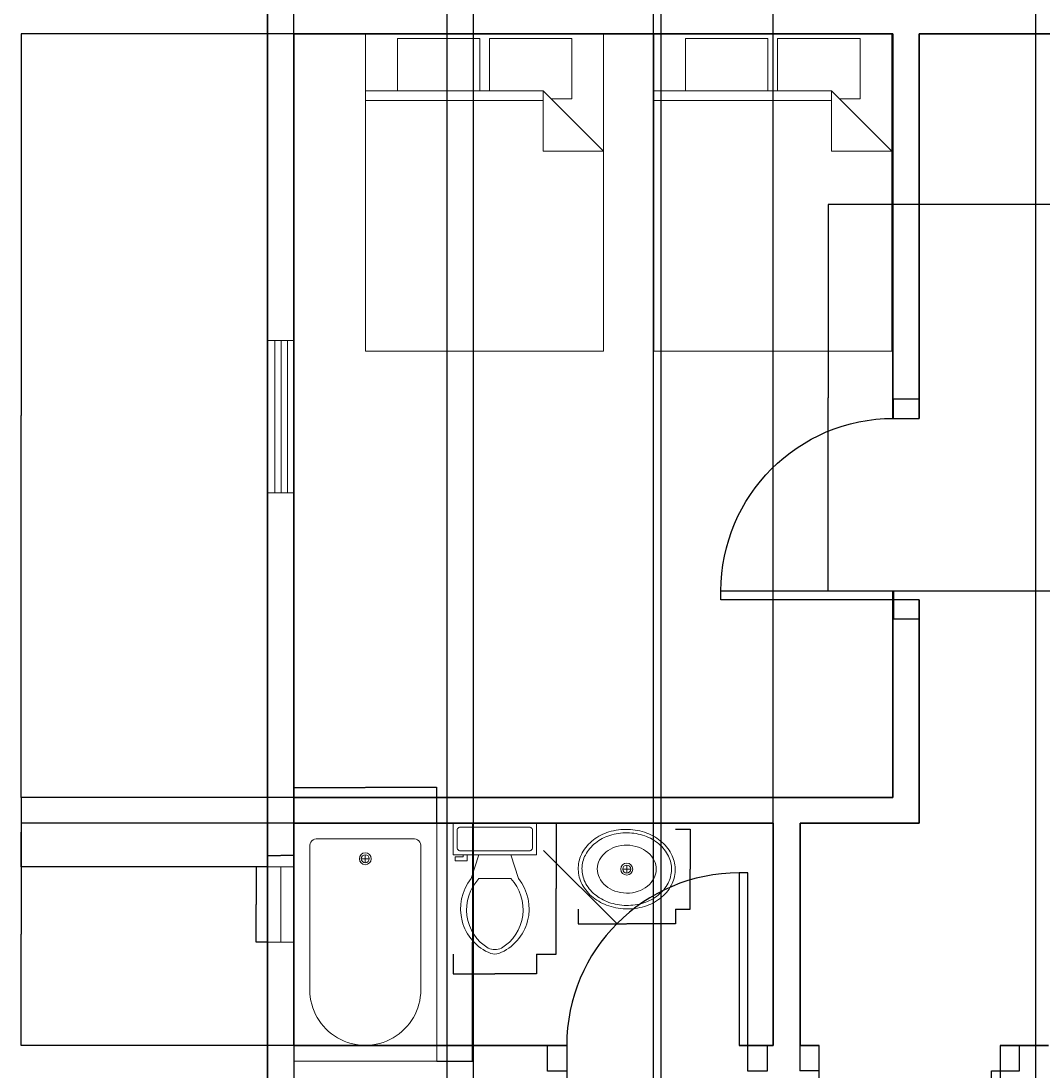
# Model space of a CAD drawing. Units: millimetres. Extents: x 31 to 27050, y -916 to 32407.
# Tile 2 of 7: x 31 to 6569, y 5664 to 12384. Entities that reach past the tile are written whole.
import ezdxf

# ---------------------------------------------------------------- set-up
doc = ezdxf.new("R2010")
doc.units = ezdxf.units.MM
for name, color, linetype, lineweight in [('A-ANNO-DIMS', 2, 'Continuous', 18), ('A-DOOR', 3, 'Continuous', 25), ('A-FLOR-FIXT', 9, 'Continuous', 18), ('A-FURN', 8, 'Continuous', 13), ('A-GLAZ', 4, 'Continuous', 18), ('A-WALL', 7, 'Continuous', 35)]:
    doc.layers.add(name, color=color, linetype=linetype, lineweight=lineweight)
doc.styles.get("Standard").update_dxf_attribs({"font": 'arial.ttf'})
doc.dimstyles.get("Standard").update_dxf_attribs({"dimtxt": 0.18, "dimasz": 0.18, "dimexe": 0.18, "dimexo": 0.0625, "dimgap": 0.09, "dimtad": 0, "dimtih": 1, "dimtoh": 1, "dimdec": 4, "dimzin": 0, "dimdsep": 46, "dimtxsty": 'Standard', "dimcen": 0.09, "dimadec": 0, "dimazin": 0, "dimtfac": 1, "dimtdec": 4, "dimtofl": 0, "dimtmove": 0, "dimatfit": 3, "dimfxl": 1, "dimtolj": 1, "dimtzin": 0, "dimarcsym": 0})

# ---------------------------------------------------------------- blocks, each defined once
blk = doc.blocks.new('Bath Tub - 26 x 60 in.')
for p, q in [((8, -18), (10, -18)), ((9, -17), (9, -19))]:
    blk.add_line(p, q)
blk.add_lwpolyline([(0, -36), (0, 0), (60, 0), (60, -36)], close=True)
for points in [[(6, -4), (42, -4)], [(4, -30), (4, -6)], [(42, -32), (6, -32)]]:
    blk.add_lwpolyline(points)
for radius in [1.5, 1]:
    blk.add_circle((9, -18), radius)
for centre, radius, start, end in [((5.75, -5.75), 1.767766999999999, 81.86989999999999, 188.1301), ((42, -18), 14, 270, 90), ((5.75, -30.25), 1.767766999999999, 171.8699, 278.1301)]:
    blk.add_arc(centre, radius, start, end)
blk = doc.blocks.new('Sink - Oval top')
for p, q in [((-1, 0), (1, 0)), ((0, 1), (0, -1))]:
    blk.add_line(p, q)
for points in [[(-12.23371880354079, 0.3941914712607968, 0.1176342565883263), (-11.46456229543957, -3.361933235489118, 0.104469279667093), (-8.878748691070427, -6.803541973650567, 0.0900157896014849), (-5.082757700676665, -9.072309807490512, 0.0819199491592185), (-0.3227280122732736, -10.01585280257211, 0.0819199491592091), (4.488169920880977, -9.380701564817912, 0.0900157896014801), (8.422342359155778, -7.36101289847943, 0.1044692796670922), (11.22435122606941, -4.093009071543406, 0.1176342565883338), (12.23371880354091, -0.3941914712607968, 0.1176342565883057), (11.46456229543992, 3.361933235488777, 0.1044692796670849), (8.878748691070427, 6.803541973650567, 0.0900157896014884), (5.082757700676324, 9.072309807490681, 0.0819199491592058), (0.3227280122732736, 10.01585280257211, 0.081919949159207), (-4.488169920880864, 9.380701564817969, 0.0900157896014802), (-8.422342359155778, 7.36101289847943, 0.1044692796670951), (-11.22435122606919, 4.093009071543633, 0.1176342565883402)], [(-11.28627986850119, 0.1590597164737346, 0.1186217001864142), (-10.51590095791209, -3.253161772358112, 0.1046781721811095), (-8.071803350560115, -6.358618019863342, 0.0895620664691738), (-4.537699193222351, -8.366971929609804, 0.0811846988912177), (-0.1289739026695997, -9.15150355811437, 0.0811846988912276), (4.300109150126218, -8.491524865184601, 0.0895620664691798), (7.889406708212618, -6.583562428127606, 0.1046781721811044), (10.42004782883111, -3.548216131892445, 0.1186217001864013), (11.28627986850119, -0.1590597164736209, 0.1186217001863945), (10.51590095791221, 3.253161772357998, 0.1046781721811069), (8.071803350560115, 6.358618019863342, 0.0895620664691756), (4.537699193222124, 8.366971929609917, 0.081184698891216), (0.1289739026695997, 9.151503558114428, 0.0811846988912142), (-4.300109150125877, 8.491524865184829, 0.0895620664691747), (-7.889406708212618, 6.583562428127606, 0.1046781721811045), (-10.42004782883111, 3.548216131892445, 0.1186217001863946)], [(-7.420452389032902, 0.0829876781601797, 0.1182825673856775), (-6.907065465214486, -2.1674649380775, 0.1046074595377274), (-5.294791470712084, -4.209988192029413, 0.0897179636260996), (-2.966599981142508, -5.528122152688069, 0.0814360825277113), (-0.0675135187855176, -6.036810076758797, 0.0814360825277218), (2.84222437824053, -5.593085960977873, 0.0897179636261315), (5.199312936802016, -4.327350491993342, 0.1046074595376878), (6.85686365682659, -2.321395784920355, 0.1182825673856714), (7.420452389033016, -0.0829876781601797, 0.1182825673856961), (6.907065465214486, 2.167464938077614, 0.1046074595377135), (5.294791470712084, 4.209988192029413, 0.0897179636261265), (2.966599981142621, 5.528122152687842, 0.0814360825277426), (0.0675135187855176, 6.036810076758797, 0.0814360825277225), (-2.842224378240644, 5.593085960977873, 0.0897179636261212), (-5.199312936802016, 4.327350491993342, 0.1046074595377049), (-6.856863656826476, 2.321395784920355, 0.1182825673856712)]]:
    blk.add_lwpolyline(points, format="xyb", close=True)
for radius in [1.5, 1]:
    blk.add_circle((0, 0), radius)
blk = doc.blocks.new('Toilet - top')
for p, q in [((9.5, -6), (9.5, -2)), ((-10, -8.5), (-8, -8.5)), ((-10, -9.5), (-10, -8.5)), ((-7, -9.5), (-10, -9.5)), ((-8, -8.5), (-8, -8)), ((-7, -8), (-7, -9.5)), ((-4, -8), (-6, -14)), ((4, -8), (6, -14)), ((4, -14), (-4, -14))]:
    blk.add_line(p, q)
blk.add_lwpolyline([(10.5, -8), (10.5, 0), (-10.5, 0), (-10.5, -8)], close=True)
for points in [[(-9.5, -2), (-9.5, -6)], [(8.5, -1), (-8.5, -1)], [(-8.5, -7), (8.5, -7)]]:
    blk.add_lwpolyline(points)
for centre, radius, start, end in [((-8.625, -1.875), 0.8838834999999999, 81.86989999999999, 188.1301), ((8.625, -1.875), 0.8838834999999999, 351.8699, 98.13009999999998), ((-8.625, -6.125), 0.8838834999999999, 171.869898, 278.1301), ((8.625, -6.125), 0.8838834999999999, 261.8699, 8.130099999999993), ((3.519562435188956, -21.58049502388982), 12.16902005083646, 141.4691096810948, 247.9714346835576), ((4.199957580658807, -21.81740929088453), 11.3291791325804, 136.3677254423718, 238.946823937405), ((-3.519499936778316, -21.58047137067522), 12.16903423757823, 292.0284332733152, 38.53070636800453), ((-4.199890672038477, -21.81738596564128), 11.32918622148567, 301.0530065773863, 43.63209216694732), ((2.09660981727e-05, -27.87646475467881), 4, 245.7318247449371, 294.2681740488959), ((2.09415214183e-05, -28.99996806116075), 4, 254.8605283244437, 285.1394707718433)]:
    blk.add_arc(centre, radius, start, end)
blk = doc.blocks.new('Bed - Queen')
for p, q in [((0, -80.00003000000002), (0, 0)), ((0, 0), (59.99998999999999, 0)), ((59.99998999999999, 0), (59.99998999999999, -80.00003000000002)), ((7.99999, -1.200000000000017), (28.79998, -1.200000000000017)), ((7.99999, -14.4), (7.99999, -1.200000000000017)), ((28.79998, -1.200000000000017), (28.79998, -14.4)), ((31.19999, -1.200000000000017), (51.99999000000001, -1.200000000000017)), ((31.19999, -14.4), (31.19999, -1.200000000000017)), ((51.99999000000001, -1.200000000000017), (51.99999000000001, -16.4)), ((0, -14.4), (44.79999999999999, -14.4)), ((59.99998999999999, -29.60000000000001), (44.79999999999999, -14.4)), ((44.79999999999999, -14.4), (44.79999999999999, -29.60000000000001)), ((44.79999999999999, -16.80000000000001), (0, -16.80000000000001)), ((51.99999000000001, -16.4), (46.79936, -16.4)), ((44.79999999999999, -29.60000000000001), (59.99998999999999, -29.60000000000001)), ((59.99998999999999, -80.00003000000002), (0, -80.00003000000002))]:
    blk.add_line(p, q)
blk = doc.blocks.new('Window - Wood Frame 36 in. Wide plan')
for p, q in [((0, 6), (0, 0)), ((36, 6), (36, 0)), ((0, 4.5), (36, 4.5)), ((0, 3), (36, 3)), ((0, 1.5), (36, 1.5))]:
    blk.add_line(p, q)
blk = doc.blocks.new('DOOR-SINGLE-1104')
for p, q in [((56.41678681898429, 1104.337341461596), (-7.18501e-11, 1104.337341461596)), ((-7.18501e-11, 1104.337341461596), (-7.18501e-11, 3.638e-12)), ((56.41678681898429, 7.276e-12), (56.41678681898429, 1104.337341461596)), ((-1226.913698425656, -163.8831223050438), (-1226.913698425656, 3.638e-12)), ((-1104.337341461589, 3.638e-12), (-1226.913698425656, 7.276e-12)), ((-1104.337341461589, 3.638e-12), (-1104.337341461589, -163.8831223050438)), ((-7.18501e-11, 3.638e-12), (56.41678681898429, 7.276e-12)), ((56.41678681898429, -163.8831223050438), (56.41678681898429, 3.638e-12)), ((56.41678681898429, 3.638e-12), (178.9931437830519, 3.638e-12)), ((178.9931437830519, 3.638e-12), (178.9931437830519, -163.8831223050438)), ((-1104.337341461589, -163.8831223050438), (-1226.913698425656, -163.8831223050438)), ((178.9931437830519, -163.8831223050438), (56.41678681898429, -163.8831223050438))]:
    blk.add_line(p, q)
blk.add_arc((0, 3.638e-12), 1104.337341461589, 90, 180)
blk = doc.blocks.new('WIN-BATH-482-FRAMED')
for p, q in [((-2.274e-13, -9.095e-13), (-168.3506507106942, -9.095e-13)), ((-168.3506507106942, -9.095e-13), (-168.3506507106942, -482.3297634273203)), ((-84.17532535534656, -482.3297634273203), (-84.17532535534723, -9.095e-13)), ((-168.3506507106942, -482.3297634273203), (1.1369e-12, -482.3297634273195)), ((1.1369e-12, -482.3297634273195), (-84.17532535534656, -482.3297634273203))]:
    blk.add_line(p, q)
blk = doc.blocks.new('*D22')
at = {"layer": 'A-ANNO-DIMS', "color": 0, "lineweight": -2, "transparency": 16777216}
for p, q in [((2692.835147825165, 7250.543705129638), (2921.552647825165, 7250.543705129638)), ((2921.372647825165, 7250.363705129638), (2921.372647825165, 6488.725608267428)), ((2921.372647825165, 5726.723705129637), (2921.372647825165, 6488.361801991849)), ((2692.835147825164, 5726.543705129636), (2921.552647825165, 5726.543705129636))]:
    blk.add_line(p, q, dxfattribs=at)
at = {"layer": 'A-ANNO-DIMS', "color": 0, "transparency": 16777216}
for points in [[(2921.342647825165, 7250.363705129638), (2921.402647825165, 7250.363705129638), (2921.372647825165, 7250.543705129638)], [(2921.342647825165, 5726.723705129637), (2921.402647825166, 5726.723705129637), (2921.372647825165, 5726.543705129636)]]:
    blk.add_solid(points, dxfattribs=at)
at = {"layer": 'Defpoints', "color": 0, "transparency": 16777216}
for p in [(2692.772647825165, 7250.543705129638), (2692.772647825164, 5726.543705129636), (2921.372647825165, 5726.543705129636)]:
    blk.add_point(p, dxfattribs=at)
at = {"layer": 'A-ANNO-DIMS', "color": 0, "transparency": 16777216, "insert": (2921.372647825167, 6488.543705129636), "char_height": 0.18, "attachment_point": 5}
blk.add_mtext('\\A1;TUB 1524 TYP.', dxfattribs=at)
blk = doc.blocks.new('*D23')
at = {"layer": 'A-ANNO-DIMS', "color": 0, "lineweight": -2, "transparency": 16777216}
for p, q in [((1778.372647825164, 7250.606205129635), (1778.372647825164, 7479.323705129636)), ((1778.552647825164, 7479.143705129636), (2234.974632818343, 7479.143705129636)), ((2692.592647825164, 7479.143705129636), (2236.170662831986, 7479.143705129636)), ((2692.772647825164, 7250.606205129635), (2692.772647825164, 7479.323705129636))]:
    blk.add_line(p, q, dxfattribs=at)
at = {"layer": 'A-ANNO-DIMS', "color": 0, "transparency": 16777216}
for points in [[(1778.552647825164, 7479.173705129635), (1778.552647825164, 7479.113705129636), (1778.372647825164, 7479.143705129636)], [(2692.592647825164, 7479.173705129635), (2692.592647825164, 7479.113705129636), (2692.772647825164, 7479.143705129636)]]:
    blk.add_solid(points, dxfattribs=at)
at = {"layer": 'Defpoints', "color": 0, "transparency": 16777216}
for p in [(2692.772647825164, 7479.143705129636), (1778.372647825164, 7250.543705129635), (2692.772647825164, 7250.543705129635)]:
    blk.add_point(p, dxfattribs=at)
at = {"layer": 'A-ANNO-DIMS', "color": 0, "transparency": 16777216, "insert": (2235.572647825164, 7479.143705129636), "char_height": 0.18, "attachment_point": 5}
blk.add_mtext('\\A1;914 TYP.', dxfattribs=at)
blk = doc.blocks.new('*D24')
at = {"layer": 'A-ANNO-DIMS', "color": 0, "lineweight": -2, "transparency": 16777216}
for p, q in [((3598.273899107064, 6699.857202883667), (3598.273899107064, 6606.20079617063)), ((4221.866610527318, 6699.857202883667), (4221.866610527318, 6606.20079617063)), ((3598.453899107064, 6606.38079617063), (3909.063986058665, 6606.38079617063)), ((4221.686610527318, 6606.38079617063), (3911.076523575718, 6606.38079617063))]:
    blk.add_line(p, q, dxfattribs=at)
at = {"layer": 'A-ANNO-DIMS', "color": 0, "transparency": 16777216}
for points in [[(3598.453899107064, 6606.41079617063), (3598.453899107064, 6606.35079617063), (3598.273899107064, 6606.38079617063)], [(4221.686610527318, 6606.41079617063), (4221.686610527318, 6606.35079617063), (4221.866610527318, 6606.38079617063)]]:
    blk.add_solid(points, dxfattribs=at)
at = {"layer": 'Defpoints', "color": 0, "transparency": 16777216}
for p in [(3598.273899107064, 6699.919702883668), (4221.866610527318, 6699.919702883668), (4221.866610527318, 6606.38079617063)]:
    blk.add_point(p, dxfattribs=at)
at = {"layer": 'A-ANNO-DIMS', "color": 0, "transparency": 16777216, "insert": (3910.070254817191, 6606.38079617063), "char_height": 0.18, "attachment_point": 5}
blk.add_mtext('\\A1;BASIN 624 TYP.', dxfattribs=at)
blk = doc.blocks.new('*D25')
at = {"layer": 'A-ANNO-DIMS', "color": 0, "lineweight": -2, "transparency": 16777216}
for p, q in [((4221.92911052732, 7211.389116326902), (4315.585517240361, 7211.389116326902)), ((4315.40551724036, 7211.209116326902), (4315.40551724036, 6955.836312743077)), ((4315.40551724036, 6700.099702883672), (4315.40551724036, 6955.472506467497)), ((4221.92911052732, 6699.919702883672), (4315.585517240361, 6699.919702883672))]:
    blk.add_line(p, q, dxfattribs=at)
at = {"layer": 'A-ANNO-DIMS', "color": 0, "transparency": 16777216}
for points in [[(4315.375517240361, 7211.209116326902), (4315.43551724036, 7211.209116326902), (4315.40551724036, 7211.389116326902)], [(4315.375517240361, 6700.099702883672), (4315.43551724036, 6700.099702883672), (4315.40551724036, 6699.919702883672)]]:
    blk.add_solid(points, dxfattribs=at)
at = {"layer": 'Defpoints', "color": 0, "transparency": 16777216}
for p in [(4221.86661052732, 7211.389116326902), (4315.40551724036, 7211.389116326902), (4221.86661052732, 6699.919702883672)]:
    blk.add_point(p, dxfattribs=at)
at = {"layer": 'A-ANNO-DIMS', "color": 0, "transparency": 16777216, "insert": (4315.405517240361, 6955.654409605284), "char_height": 0.18, "attachment_point": 5}
blk.add_mtext('\\A1;511 TYP.', dxfattribs=at)
blk = doc.blocks.new('*D26')
at = {"layer": 'A-ANNO-DIMS', "color": 0, "lineweight": -2, "transparency": 16777216}
for p, q in [((3332.083189867999, 7250.543705129638), (3458.106880059174, 7250.543705129638)), ((3457.926880059174, 7250.363705129638), (3457.926880059175, 6831.039535461012)), ((3457.926880059175, 6411.349103855144), (3457.926880059175, 6830.673273523768)), ((3332.083189867999, 6411.169103855144), (3458.106880059175, 6411.169103855144))]:
    blk.add_line(p, q, dxfattribs=at)
at = {"layer": 'A-ANNO-DIMS', "color": 0, "transparency": 16777216}
for points in [[(3457.896880059174, 7250.363705129638), (3457.956880059175, 7250.363705129638), (3457.926880059174, 7250.543705129638)], [(3457.896880059175, 6411.349103855144), (3457.956880059175, 6411.349103855144), (3457.926880059175, 6411.169103855144)]]:
    blk.add_solid(points, dxfattribs=at)
at = {"layer": 'Defpoints', "color": 0, "transparency": 16777216}
for p in [(3332.020689867999, 7250.543705129638), (3457.926880059174, 7250.543705129638), (3332.020689867999, 6411.169103855144)]:
    blk.add_point(p, dxfattribs=at)
at = {"layer": 'A-ANNO-DIMS', "color": 0, "transparency": 16777216, "insert": (3457.926880059176, 6830.856404492388), "char_height": 0.18, "attachment_point": 5}
blk.add_mtext('\\A1;WC 839 TYP.', dxfattribs=at)
blk = doc.blocks.new('*D27')
at = {"layer": 'A-ANNO-DIMS', "color": 0, "lineweight": -2, "transparency": 16777216}
for p, q in [((2798.620689867997, 6411.10660385514), (2798.620689867997, 6285.082913663965)), ((3332.020689867997, 6411.10660385514), (3332.020689867997, 6285.082913663965)), ((2798.800689867997, 6285.262913663966), (3064.722674861176, 6285.262913663966)), ((3331.840689867997, 6285.262913663966), (3065.918704874818, 6285.262913663966))]:
    blk.add_line(p, q, dxfattribs=at)
at = {"layer": 'A-ANNO-DIMS', "color": 0, "transparency": 16777216}
for points in [[(2798.800689867997, 6285.292913663965), (2798.800689867997, 6285.232913663965), (2798.620689867997, 6285.262913663966)], [(3331.840689867997, 6285.292913663965), (3331.840689867997, 6285.232913663965), (3332.020689867997, 6285.262913663966)]]:
    blk.add_solid(points, dxfattribs=at)
at = {"layer": 'Defpoints', "color": 0, "transparency": 16777216}
for p in [(2798.620689867997, 6411.16910385514), (3332.020689867997, 6411.16910385514), (3332.020689867997, 6285.262913663966)]:
    blk.add_point(p, dxfattribs=at)
at = {"layer": 'A-ANNO-DIMS', "color": 0, "transparency": 16777216, "insert": (3065.320689867997, 6285.262913663966), "char_height": 0.18, "attachment_point": 5}
blk.add_mtext('\\A1;533 TYP.', dxfattribs=at)
blk = doc.blocks.new('*D42')
at = {"layer": 'A-ANNO-DIMS', "color": 0, "lineweight": -2, "transparency": 16777216}
for p, q in [((1609.959497114469, 6971.117434470525), (1537.492532600372, 6971.117434470525)), ((1537.672532600373, 6970.937434470525), (1537.672532600373, 6730.135683725489)), ((1537.672532600373, 6488.967671043207), (1537.672532600373, 6729.769421788244)), ((1609.959497114469, 6488.787671043207), (1537.492532600373, 6488.787671043207))]:
    blk.add_line(p, q, dxfattribs=at)
at = {"layer": 'A-ANNO-DIMS', "color": 0, "transparency": 16777216}
for points in [[(1537.642532600373, 6970.937434470525), (1537.702532600373, 6970.937434470525), (1537.672532600373, 6971.117434470525)], [(1537.642532600373, 6488.967671043207), (1537.702532600373, 6488.967671043207), (1537.672532600373, 6488.787671043207)]]:
    blk.add_solid(points, dxfattribs=at)
at = {"layer": 'Defpoints', "color": 0, "transparency": 16777216}
for p in [(1537.672532600373, 6971.117434470525), (1610.021997114469, 6971.117434470525), (1610.021997114469, 6488.787671043207)]:
    blk.add_point(p, dxfattribs=at)
at = {"layer": 'A-ANNO-DIMS', "color": 0, "transparency": 16777216, "insert": (1537.672532600374, 6729.952552756865), "char_height": 0.18, "attachment_point": 5}
blk.add_mtext('\\A1;FRAMED WINDOW 482 TYP.', dxfattribs=at)
blk = doc.blocks.new('*D43')
at = {"layer": 'A-ANNO-DIMS', "color": 0, "lineweight": -2, "transparency": 16777216}
for p, q in [((1610.021997114469, 6971.179934470523), (1610.021997114469, 7043.64689898462)), ((1610.201997114469, 7043.46689898462), (1693.607779495737, 7043.46689898462)), ((1778.192647825164, 7043.46689898462), (1694.786865443895, 7043.46689898462)), ((1778.372647825164, 6971.179934470523), (1778.372647825164, 7043.64689898462))]:
    blk.add_line(p, q, dxfattribs=at)
at = {"layer": 'A-ANNO-DIMS', "color": 0, "transparency": 16777216}
for points in [[(1610.201997114469, 7043.49689898462), (1610.201997114469, 7043.43689898462), (1610.021997114469, 7043.46689898462)], [(1778.192647825164, 7043.49689898462), (1778.192647825164, 7043.43689898462), (1778.372647825164, 7043.46689898462)]]:
    blk.add_solid(points, dxfattribs=at)
at = {"layer": 'Defpoints', "color": 0, "transparency": 16777216}
for p in [(1778.372647825164, 7043.46689898462), (1610.021997114469, 6971.117434470523), (1778.372647825164, 6971.117434470523)]:
    blk.add_point(p, dxfattribs=at)
at = {"layer": 'A-ANNO-DIMS', "color": 0, "transparency": 16777216, "insert": (1694.197322469817, 7043.46689898462), "char_height": 0.18, "attachment_point": 5}
blk.add_mtext('\\A1;168 TYP.', dxfattribs=at)
blk = doc.blocks.new('*D57')
at = {"layer": 'A-ANNO-DIMS', "color": 0, "lineweight": -2, "transparency": 16777216}
for p, q in [((1778.310148000001, 12301.860549), (30.84199699999932, 12301.860549)), ((31.02199699999948, 12301.68054900001), (31.02199700000003, 9858.325591137795)), ((31.02199700000057, 7414.606827000004), (31.02199700000003, 9857.961784862217)), ((1778.310148000001, 7414.426827000004), (30.8419970000004, 7414.426827000004))]:
    blk.add_line(p, q, dxfattribs=at)
at = {"layer": 'A-ANNO-DIMS', "color": 0, "transparency": 16777216}
for points in [[(30.99199699999948, 12301.68054900001), (31.05199699999948, 12301.68054900001), (31.02199699999948, 12301.860549)], [(30.99199700000057, 7414.606827000004), (31.05199700000057, 7414.606827000004), (31.02199700000057, 7414.426827000004)]]:
    blk.add_solid(points, dxfattribs=at)
at = {"layer": 'Defpoints', "color": 0, "transparency": 16777216}
for p in [(31.02199699999948, 12301.860549), (1778.372648000001, 12301.860549), (1778.372648000001, 7414.426827000004)]:
    blk.add_point(p, dxfattribs=at)
at = {"layer": 'A-ANNO-DIMS', "color": 0, "transparency": 16777216, "insert": (31.02199700000281, 9858.143688000006), "char_height": 0.18, "attachment_point": 5}
blk.add_mtext('\\A1;4887', dxfattribs=at)
blk = doc.blocks.new('*D58')
at = {"layer": 'A-ANNO-DIMS', "color": 0, "lineweight": -2, "transparency": 16777216}
for p, q in [((1778.310148000001, 7250.543705000004), (30.84199699999976, 7250.543705000004)), ((31.02199699999987, 7250.363705000004), (31.02199700000003, 6539.219446529336)), ((31.02199700000019, 5827.711259000002), (31.02199700000003, 6538.855517470672)), ((1778.310148000001, 5827.531259000002), (30.84199700000007, 5827.531259000002))]:
    blk.add_line(p, q, dxfattribs=at)
at = {"layer": 'A-ANNO-DIMS', "color": 0, "transparency": 16777216}
for points in [[(30.99199699999987, 7250.363705000004), (31.05199699999988, 7250.363705000004), (31.02199699999987, 7250.543705000004)], [(30.99199700000019, 5827.711259000002), (31.05199700000019, 5827.711259000002), (31.02199700000019, 5827.531259000002)]]:
    blk.add_solid(points, dxfattribs=at)
at = {"layer": 'Defpoints', "color": 0, "transparency": 16777216}
for p in [(31.02199699999987, 7250.543705000004), (1778.372648000001, 7250.543705000004), (1778.372648000001, 5827.531259000002)]:
    blk.add_point(p, dxfattribs=at)
at = {"layer": 'A-ANNO-DIMS', "color": 0, "transparency": 16777216, "insert": (31.02199700000188, 6539.037482000002), "char_height": 0.18, "attachment_point": 5}
blk.add_mtext('\\A1;1423', dxfattribs=at)
blk = doc.blocks.new('*D61')
at = {"layer": 'A-ANNO-DIMS', "color": 0, "lineweight": -2, "transparency": 16777216}
for p, q in [((1778.372648, 7250.606205), (1778.372648000001, 32406.711259)), ((1778.552648000001, 32406.531259), (3312.109331318556, 32406.531259)), ((4846.592413000001, 32406.531259), (3313.035729681448, 32406.531259)), ((4846.772413, 7250.606205), (4846.772413000001, 32406.711259))]:
    blk.add_line(p, q, dxfattribs=at)
at = {"layer": 'A-ANNO-DIMS', "color": 0, "transparency": 16777216}
for points in [[(1778.552648000001, 32406.561259), (1778.552648000001, 32406.501259), (1778.372648000001, 32406.531259)], [(4846.592413000001, 32406.561259), (4846.592413000001, 32406.501259), (4846.772413000001, 32406.531259)]]:
    blk.add_solid(points, dxfattribs=at)
at = {"layer": 'Defpoints', "color": 0, "transparency": 16777216}
for p in [(4846.772413000001, 32406.531259), (1778.372648, 7250.543705), (4846.772413, 7250.543705)]:
    blk.add_point(p, dxfattribs=at)
at = {"layer": 'A-ANNO-DIMS', "color": 0, "transparency": 16777216, "insert": (3312.572530500002, 32406.531259), "char_height": 0.18, "attachment_point": 5}
blk.add_mtext('\\A1;3068.4', dxfattribs=at)
blk = doc.blocks.new('*D64')
at = {"layer": 'A-ANNO-DIMS', "color": 0, "lineweight": -2, "transparency": 16777216}
for p, q in [((6778.040612000004, 11210.336516), (5198.923112000002, 11210.336516)), ((5199.103112000003, 11210.156516), (5199.103112000003, 9972.897271637792)), ((5199.103112000003, 8735.274221000001), (5199.103112000003, 9972.533465362214)), ((6778.040612000004, 8735.094221000001), (5198.923112000003, 8735.094221000001))]:
    blk.add_line(p, q, dxfattribs=at)
at = {"layer": 'A-ANNO-DIMS', "color": 0, "transparency": 16777216}
for points in [[(5199.073112000003, 11210.156516), (5199.133112000002, 11210.156516), (5199.103112000003, 11210.336516)], [(5199.073112000004, 8735.274221000001), (5199.133112000003, 8735.274221000001), (5199.103112000003, 8735.094221000001)]]:
    blk.add_solid(points, dxfattribs=at)
at = {"layer": 'Defpoints', "color": 0, "transparency": 16777216}
for p in [(5199.103112000003, 11210.336516), (6778.103112000003, 11210.336516), (6778.103112000003, 8735.094221000001)]:
    blk.add_point(p, dxfattribs=at)
at = {"layer": 'A-ANNO-DIMS', "color": 0, "transparency": 16777216, "insert": (5199.103112000005, 9972.7153685), "char_height": 0.18, "attachment_point": 5}
blk.add_mtext('\\A1;2475', dxfattribs=at)
blk = doc.blocks.new('*D69')
at = {"layer": 'A-ANNO-DIMS', "color": 0, "lineweight": -2, "transparency": 16777216}
for p, q in [((2757.340836, 14467.362437), (2757.340835999999, -915.5318640000004)), ((4128.594056999999, 14467.362437), (4128.594056999999, -915.5318640000004)), ((2757.520835999999, -915.3518639999999), (3442.512289610504, -915.3518639999999)), ((4128.414056999999, -915.3518639999999), (3443.422603389495, -915.3518639999999))]:
    blk.add_line(p, q, dxfattribs=at)
at = {"layer": 'A-ANNO-DIMS', "color": 0, "transparency": 16777216}
for points in [[(2757.520835999999, -915.321864), (2757.520835999999, -915.381864), (2757.340835999999, -915.3518639999999)], [(4128.414056999999, -915.321864), (4128.414056999999, -915.381864), (4128.594056999999, -915.3518639999999)]]:
    blk.add_solid(points, dxfattribs=at)
at = {"layer": 'Defpoints', "color": 0, "transparency": 16777216}
for p in [(2757.340836, 14467.424937), (4128.594056999999, 14467.424937), (4128.594056999999, -915.3518639999999)]:
    blk.add_point(p, dxfattribs=at)
at = {"layer": 'A-ANNO-DIMS', "color": 0, "transparency": 16777216, "insert": (3442.967446499999, -915.3518639999999), "char_height": 0.18, "attachment_point": 5}
blk.add_mtext('\\A1;1371.3', dxfattribs=at)
blk = doc.blocks.new('*D70')
at = {"layer": 'A-ANNO-DIMS', "color": 0, "lineweight": -2, "transparency": 16777216}
for p, q in [((4128.594056999999, 14467.362437), (4128.594056999999, -915.5318640000004)), ((6528.594057000001, 14467.362437), (6528.594056999999, -915.5318640000004)), ((4128.774057, -915.3518639999999), (5328.234056999999, -915.3518639999999)), ((6528.414056999999, -915.3518639999999), (5328.954056999999, -915.3518639999999))]:
    blk.add_line(p, q, dxfattribs=at)
at = {"layer": 'A-ANNO-DIMS', "color": 0, "transparency": 16777216}
for points in [[(4128.774057, -915.321864), (4128.774057, -915.381864), (4128.594056999999, -915.3518639999999)], [(6528.414056999999, -915.321864), (6528.414056999999, -915.381864), (6528.594056999999, -915.3518639999999)]]:
    blk.add_solid(points, dxfattribs=at)
at = {"layer": 'Defpoints', "color": 0, "transparency": 16777216}
for p in [(4128.594056999999, 14467.424937), (6528.594057000001, 14467.424937), (6528.594056999999, -915.3518639999999)]:
    blk.add_point(p, dxfattribs=at)
at = {"layer": 'A-ANNO-DIMS', "color": 0, "transparency": 16777216, "insert": (5328.594057, -915.3518639999999), "char_height": 0.18, "attachment_point": 5}
blk.add_mtext('\\A1;2400', dxfattribs=at)
blk = doc.blocks.new('*D84')
at = {"layer": 'A-ANNO-DIMS', "color": 0, "lineweight": -2, "transparency": 16777216}
for p, q in [((1778.310148000001, 7414.426827000004), (30.84199699999995, 7414.426827000004)), ((31.02199699999998, 7414.246827000003), (31.02199700000003, 7192.954095029334)), ((31.02199700000008, 6971.297434000004), (31.02199700000003, 7192.590165970671)), ((1609.959497000001, 6971.117434000004), (30.84199700000004, 6971.117434000004))]:
    blk.add_line(p, q, dxfattribs=at)
at = {"layer": 'A-ANNO-DIMS', "color": 0, "transparency": 16777216}
for points in [[(30.99199699999998, 7414.246827000003), (31.05199699999998, 7414.246827000003), (31.02199699999998, 7414.426827000004)], [(30.99199700000008, 6971.297434000004), (31.05199700000008, 6971.297434000004), (31.02199700000008, 6971.117434000004)]]:
    blk.add_solid(points, dxfattribs=at)
at = {"layer": 'Defpoints', "color": 0, "transparency": 16777216}
for p in [(31.02199699999998, 7414.426827000004), (1778.372648000001, 7414.426827000004), (1610.021997000001, 6971.117434000004)]:
    blk.add_point(p, dxfattribs=at)
at = {"layer": 'A-ANNO-DIMS', "color": 0, "transparency": 16777216, "insert": (31.02199700000206, 7192.772130500002), "char_height": 0.18, "attachment_point": 5}
blk.add_mtext('\\A1;443.3', dxfattribs=at)
blk = doc.blocks.new('*D92')
at = {"layer": 'A-ANNO-DIMS', "color": 0, "lineweight": -2, "transparency": 16777216}
for p, q in [((1778.372648, 5827.468759000001), (1778.372647999999, -915.5318640000004)), ((3525.344535, 5827.468759000001), (3525.344535, -915.5318640000004)), ((1778.552647999999, -915.3518639999999), (2651.508291363575, -915.3518639999999)), ((3525.164535, -915.3518639999999), (2652.208891636425, -915.3518639999999))]:
    blk.add_line(p, q, dxfattribs=at)
at = {"layer": 'A-ANNO-DIMS', "color": 0, "transparency": 16777216}
for points in [[(1778.552647999999, -915.321864), (1778.552647999999, -915.381864), (1778.372647999999, -915.3518639999999)], [(3525.164535, -915.321864), (3525.164535, -915.381864), (3525.344535, -915.3518639999999)]]:
    blk.add_solid(points, dxfattribs=at)
at = {"layer": 'Defpoints', "color": 0, "transparency": 16777216}
for p in [(1778.372648, 5827.531259), (3525.344535, 5827.531259), (3525.344535, -915.3518639999999)]:
    blk.add_point(p, dxfattribs=at)
at = {"layer": 'A-ANNO-DIMS', "color": 0, "transparency": 16777216, "insert": (2651.8585915, -915.3518639999999), "char_height": 0.18, "attachment_point": 5}
blk.add_mtext('\\A1;1747', dxfattribs=at)
blk = doc.blocks.new('*D93')
at = {"layer": 'A-ANNO-DIMS', "color": 0, "lineweight": -2, "transparency": 16777216}
for p, q in [((2925.691486, 14303.479314), (2925.691486, -915.5318640000004)), ((4078.94748, 14303.479314), (4078.947479999999, -915.5318640000004)), ((2925.871485999999, -915.3518639999999), (3501.864326110504, -915.3518639999999)), ((4078.767479999998, -915.3518639999999), (3502.774639889495, -915.3518639999999))]:
    blk.add_line(p, q, dxfattribs=at)
at = {"layer": 'A-ANNO-DIMS', "color": 0, "transparency": 16777216}
for points in [[(2925.871485999999, -915.321864), (2925.871485999999, -915.381864), (2925.691486, -915.3518639999999)], [(4078.767479999998, -915.321864), (4078.767479999998, -915.381864), (4078.947479999999, -915.3518639999999)]]:
    blk.add_solid(points, dxfattribs=at)
at = {"layer": 'Defpoints', "color": 0, "transparency": 16777216}
for p in [(2925.691486, 14303.541814), (4078.94748, 14303.541814), (4078.947479999999, -915.3518639999999)]:
    blk.add_point(p, dxfattribs=at)
at = {"layer": 'A-ANNO-DIMS', "color": 0, "transparency": 16777216, "insert": (3502.319482999999, -915.3518639999999), "char_height": 0.18, "attachment_point": 5}
blk.add_mtext('\\A1;1153.3', dxfattribs=at)
blk = doc.blocks.new('*D95')
at = {"layer": 'A-ANNO-DIMS', "color": 0, "lineweight": -2, "transparency": 16777216}
for p, q in [((3377.522847247268, 7074.377110152927), (3377.702847247268, 7074.377110152926)), ((3377.702847247268, 7074.377110152926), (3847.067442586853, 6606.936933490977)), ((4629.591876, 5827.531259000001), (4629.771876, 5827.531259)), ((4629.681876000001, 5827.441259000001), (4629.681875999998, 5827.621259000001))]:
    blk.add_line(p, q, dxfattribs=at)
at = {"layer": 'A-ANNO-DIMS', "color": 0, "transparency": 16777216}
blk.add_solid([(3847.088612168682, 6606.958190226501), (3847.046273005023, 6606.915676755453), (3847.194983000001, 6606.809916)], dxfattribs=at)
at = {"layer": 'Defpoints', "color": 0, "transparency": 16777216}
for p in [(3847.194983000001, 6606.809916), (4629.681876, 5827.531259000001)]:
    blk.add_point(p, dxfattribs=at)
at = {"layer": 'A-ANNO-DIMS', "color": 0, "transparency": 16777216, "insert": (3376.708242881647, 7074.377110152927), "char_height": 0.18, "attachment_point": 5}
blk.add_mtext('\\A1;28X R1104.3', dxfattribs=at)

msp = doc.modelspace()

# ---------------------------------------------------------------- linework, layer by layer
at = {"layer": 'A-DOOR'}
for p, q in [((5617.824553716266, 8556.807120053505), (5781.707676021313, 8556.807120053505)), ((5019.966376369207, 5827.531258671735), (5141.437222462371, 5827.531258671735)), ((6424.767707707011, 5663.648136366686), (6424.767707707011, 5827.531258671734))]:
    msp.add_line(p, q, dxfattribs=at)
at = {"layer": 'A-WALL'}
for p, q in [((1610.021997114469, 744.3803777755929), (1610.021997114469, 12465.74367114627)), ((5613.357025310619, 12301.86054884122), (1778.372647825163, 12301.86054884122)), ((1778.372647825163, 5827.531258671735), (1778.372647825163, 12301.86054884122)), ((5613.357025310619, 12301.86054884122), (5613.357025310619, 9840.128568706263)), ((5781.707676021313, 12301.86054884122), (5781.707676021314, 9840.137605298149)), ((8211.090788713413, 12301.86054884122), (5781.707676021313, 12301.86054884121)), ((5613.357025310619, 8735.80026383663), (5613.357025310619, 7414.426827434685)), ((5781.707676021315, 8679.383477017574), (5781.707676021314, 7331.275946538546)), ((4846.772413104511, 7414.426827434685), (1778.372647825163, 7414.426827434685)), ((4846.772413104511, 7414.426827434685), (4926.421654242644, 7414.426827434687)), ((5613.357025310619, 7414.426827434685), (4926.421654242644, 7414.426827434687)), ((5781.707676021314, 7250.543705129635), (5781.707676021314, 7331.275946538546)), ((4846.772413104511, 7250.543705129635), (1778.372647825163, 7250.543705129636)), ((4846.772413104512, 7250.543705129635), (4846.772413104511, 5827.531258671734)), ((5693.9203608066, 7250.543705129635), (5019.966376369208, 7250.543705129635)), ((5019.966376369208, 7250.543705129635), (5019.966376369208, 5827.531258671735)), ((5693.9203608066, 7250.543705129635), (5781.707676021314, 7250.543705129635)), ((1778.372647825163, 5827.531258671735), (3525.344534980938, 5827.531258671734)), ((4629.681876442453, 5827.531258671734), (4846.772413104512, 5827.531258671734)), ((6302.191350742941, 5827.531258671733), (6610.021997114469, 5827.531258671733))]:
    msp.add_line(p, q, dxfattribs=at)

# ---------------------------------------------------------------- block references
at = {"layer": 'A-DOOR', "extrusion": (0, 0, -1), "zscale": -1}
for p, rotation in [((-5617.82455371628, 8735.800263836558), 270.0000000000002), ((-6245.774563923957, 5663.648136366701), 180)]:
    msp.add_blockref('DOOR-SINGLE-1104', p, dxfattribs=dict(at, rotation=rotation))
at = {"layer": 'A-DOOR'}
msp.add_blockref('DOOR-SINGLE-1104', (4629.681876442521, 5827.531258671719), dxfattribs=at)
at = {"layer": 'A-FLOR-FIXT', "xscale": 25.4, "yscale": 25.4, "zscale": 25.4, "rotation": 270}
msp.add_blockref('Bath Tub - 26 x 60 in.', (2692.772647825164, 7250.543705129635), dxfattribs=at)
at = {"layer": 'A-FLOR-FIXT', "xscale": 25.4, "yscale": 25.4, "zscale": 25.4}
for name, p in [('Toilet - top', (3065.320689867997, 7250.543705129635)), ('Sink - Oval top', (3910.07025481719, 6955.654409605282))]:
    msp.add_blockref(name, p, dxfattribs=at)
at = {"layer": 'A-FURN', "xscale": 25.4, "yscale": 25.4, "zscale": 25.4}
for p in [(2237.698750248645, 12301.86054884122), (4082.975090126507, 12301.86054884122)]:
    msp.add_blockref('Bed - Queen', p, dxfattribs=at)
at = {"layer": 'A-GLAZ', "xscale": 27.11229900122799, "yscale": 27.11229900122799, "zscale": 27.11229900122799, "rotation": 90}
msp.add_blockref('Window - Wood Frame 36 in. Wide plan', (1778.372647825162, 9363.310953655888), dxfattribs=at)
at = {"layer": 'A-GLAZ'}
msp.add_blockref('WIN-BATH-482-FRAMED', (1778.372647825163, 6971.117434470523), dxfattribs=at)

# ---------------------------------------------------------------- dimensions: what is measured, and where the dimension line sits
at = {"layer": 'A-ANNO-DIMS'}
for base, p1, p2, override, picture, middle in [((4846.772413000001, 32406.531259), (1778.372648, 7250.543705), (4846.772413, 7250.543705), {"dimdec": 1, "dimlfac": 1, "dimrnd": 0, "dimzin": 0, "dimdsep": 46, "dimlunit": 2}, '*D61', (3312.572530500002, 32406.531259)), ((4128.594056999999, -915.3518639999999), (2757.340836, 14467.424937), (4128.594056999999, 14467.424937), {"dimdec": 1, "dimlfac": 1, "dimrnd": 0, "dimzin": 0, "dimdsep": 46, "dimlunit": 2}, '*D69', (3442.967446499999, -915.3518639999999)), ((6528.594056999999, -915.3518639999999), (4128.594056999999, 14467.424937), (6528.594057000001, 14467.424937), {"dimdec": 0, "dimlfac": 1, "dimrnd": 0, "dimzin": 0, "dimdsep": 46, "dimlunit": 2}, '*D70', (5328.594057, -915.3518639999999)), ((4078.947479999999, -915.3518639999999), (2925.691486, 14303.541814), (4078.94748, 14303.541814), {"dimdec": 1, "dimlfac": 1, "dimrnd": 0, "dimzin": 0, "dimdsep": 46, "dimlunit": 2}, '*D93', (3502.319482999999, -915.3518639999999)), ((3525.344535, -915.3518639999999), (1778.372648, 5827.531259), (3525.344535, 5827.531259), {"dimdec": 0, "dimlfac": 1, "dimrnd": 0, "dimzin": 0, "dimdsep": 46, "dimlunit": 2}, '*D92', (2651.8585915, -915.3518639999999))]:
    dim = msp.add_linear_dim(base=base, p1=p1, p2=p2, dimstyle='Standard', override=override, dxfattribs=at)
    dim.commit()
    dim.dimension.update_dxf_attribs({"geometry": picture, "text_midpoint": middle})
for base, p1, p2, angle, override, picture, middle in [((31.02199699999948, 12301.860549), (1778.372648, 7414.426826999999), (1778.372648, 12301.860549), 90, {"dimdec": 0, "dimlfac": 1, "dimrnd": 0, "dimzin": 0, "dimdsep": 46, "dimlunit": 2}, '*D57', (31.02199700000281, 9858.143688000006)), ((5199.103112000003, 11210.336516), (6778.103112, 8735.094221), (6778.103112, 11210.336516), 90.00000000000018, {"dimdec": 0, "dimlfac": 1, "dimrnd": 0, "dimzin": 0, "dimdsep": 46, "dimlunit": 2}, '*D64', (5199.103112000005, 9972.7153685)), ((31.02199699999998, 7414.426827000004), (1610.021997, 6971.117433999999), (1778.372648, 7414.426826999999), 90, {"dimdec": 1, "dimlfac": 1, "dimrnd": 0, "dimzin": 0, "dimdsep": 46, "dimlunit": 2}, '*D84', (31.02199700000206, 7192.772130500002)), ((31.02199699999987, 7250.543705000004), (1778.372648, 5827.531259), (1778.372648, 7250.543705), 90, {"dimdec": 0, "dimlfac": 1, "dimrnd": 0, "dimzin": 0, "dimdsep": 46, "dimlunit": 2}, '*D58', (31.02199700000188, 6539.037482000002))]:
    dim = msp.add_linear_dim(base=base, p1=p1, p2=p2, angle=angle, dimstyle='Standard', override=override, dxfattribs=at)
    dim.commit()
    dim.dimension.update_dxf_attribs({"geometry": picture, "text_midpoint": middle})
for base, p1, p2, text, picture, middle in [((2692.772647825164, 7479.143705129636), (1778.372647825164, 7250.543705129635), (2692.772647825164, 7250.543705129635), '<> TYP.', '*D23', (2235.572647825164, 7479.143705129636)), ((1778.372647825164, 7043.46689898462), (1610.021997114469, 6971.117434470523), (1778.372647825164, 6971.117434470523), '<> TYP.', '*D43', (1694.197322469817, 7043.46689898462)), ((4221.866610527318, 6606.38079617063), (3598.273899107064, 6699.919702883668), (4221.866610527318, 6699.919702883668), 'BASIN <> TYP.', '*D24', (3910.070254817191, 6606.38079617063)), ((3332.020689867997, 6285.262913663966), (2798.620689867997, 6411.16910385514), (3332.020689867997, 6411.16910385514), '<> TYP.', '*D27', (3065.320689867997, 6285.262913663966))]:
    dim = msp.add_linear_dim(base=base, p1=p1, p2=p2, text=text, dimstyle='Standard', override={"dimdec": 0, "dimlfac": 1, "dimrnd": 0, "dimzin": 0, "dimdsep": 46, "dimlunit": 2}, dxfattribs=at)
    dim.commit()
    dim.dimension.update_dxf_attribs({"geometry": picture, "text_midpoint": middle})
for base, p1, p2, angle, text, picture, middle in [((2921.372647825165, 5726.543705129636), (2692.772647825164, 7250.543705129635), (2692.772647825164, 5726.543705129635), 270, 'TUB <> TYP.', '*D22', (2921.372647825167, 6488.543705129636)), ((3457.926880059174, 7250.543705129638), (3332.020689867997, 6411.16910385514), (3332.020689867997, 7250.543705129635), 90, 'WC <> TYP.', '*D26', (3457.926880059176, 6830.856404492388)), ((4315.40551724036, 7211.389116326902), (4221.866610527318, 6699.919702883668), (4221.866610527318, 7211.389116326897), 90, '<> TYP.', '*D25', (4315.405517240361, 6955.654409605284)), ((1537.672532600373, 6971.117434470525), (1610.021997114469, 6488.787671043202), (1610.021997114469, 6971.117434470523), 90, 'FRAMED WINDOW <> TYP.', '*D42', (1537.672532600374, 6729.952552756865))]:
    dim = msp.add_linear_dim(base=base, p1=p1, p2=p2, angle=angle, text=text, dimstyle='Standard', override={"dimdec": 0, "dimlfac": 1, "dimrnd": 0, "dimzin": 0, "dimdsep": 46, "dimlunit": 2}, dxfattribs=at)
    dim.commit()
    dim.dimension.update_dxf_attribs({"geometry": picture, "text_midpoint": middle})
dim = msp.add_radius_dim(center=(4629.681876, 5827.531259000001), mpoint=(3847.194983000001, 6606.809916), text='28X <>', dimstyle='Standard', override={"dimdec": 1, "dimlfac": 1, "dimrnd": 0, "dimzin": 0, "dimdsep": 46, "dimlunit": 2}, dxfattribs=at)
dim.commit()
dim.dimension.update_dxf_attribs({"geometry": '*D95', "text_midpoint": (3376.708242881647, 7074.377110152927), "dimtype": 164})

doc.saveas('drawing.dxf')
